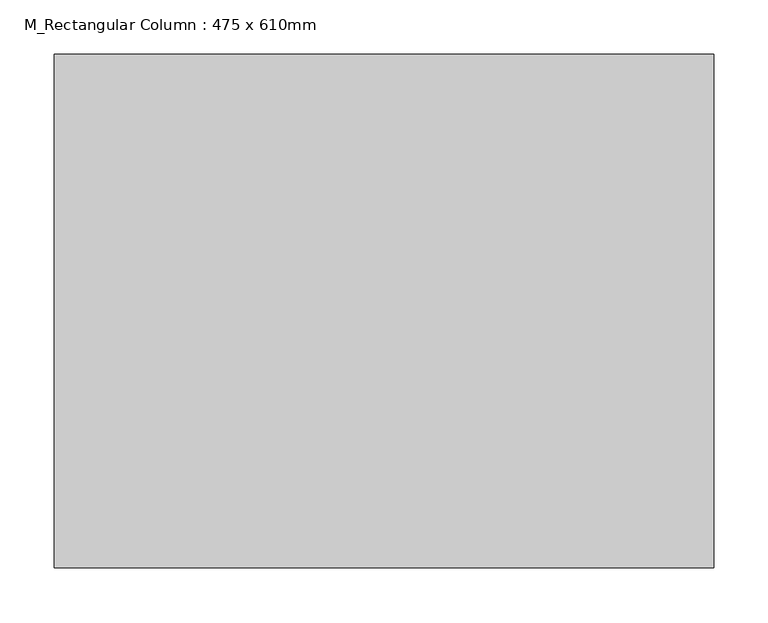
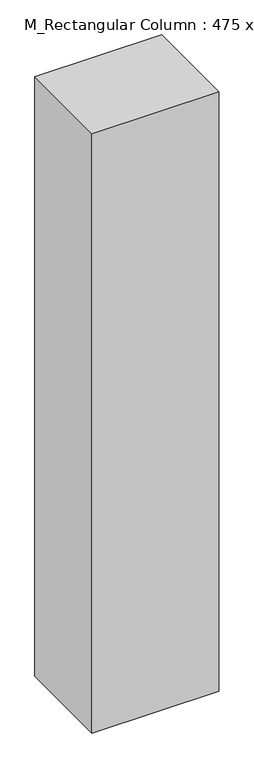
"""IFC4 building model written with IfcOpenShell, lengths in millimetres: column geometry, M_Rectangular Column : 475 x 610mm."""

from ifc_helpers import new_model, si_unit, frame, origin, place, context, project, spatial, polyline, outline, extrude, source, transform, mapped, element, save


def m_rectangular_column_475_x_610mm_d36e7488(model_context):
    return source(origin(), model_context, "Body", "SweptSolid", [
        extrude(outline(polyline([(305.0, 237.5), (305.0, -237.5), (-305.0, -237.5), (-305.0, 237.5), (305.0, 237.5)])), frame((0.0, 0.0, 3048.0), z_axis=(0.0, 0.0, 1.0), x_axis=(1.0, 0.0, 0.0)), (0.0, 0.0, 1.0), 3048.0),
    ])


if __name__ == "__main__":
    model = new_model("IFC4")
    model_context = context("Model", 3, world=origin())
    ifc_project = project(units=[si_unit("LENGTHUNIT", "METRE", prefix="MILLI")], contexts=[model_context])
    site = spatial("IfcSite", under=ifc_project)
    building = spatial("IfcBuilding", under=site)
    placement = place(None, origin())
    m_rectangular_column_475_x_610mm_shape = m_rectangular_column_475_x_610mm_d36e7488(model_context)
    element("IfcColumn", 1, ObjectType="M_Rectangular Column : 475 x 610mm", at=placement, inside=building, context=model_context, shape_type="MappedRepresentation", body=[
        mapped(m_rectangular_column_475_x_610mm_shape, transform((0.0, 0.0, 0.0), x_axis=(1.0, 0.0, 0.0), y_axis=(0.0, 1.0, 0.0), z_axis=(0.0, 0.0, 1.0))),
    ])
    save(model, "model.ifc")

# Revit data of these elements
# Type "M_Rectangular Column : 475 x 610mm"
#   Depth = 1' - 6.70079"
#   Offset Base = 0' - 0"
#   Offset Top = 0' - 0"
#   Width = 2' - 0.01575"
#   Material = none
